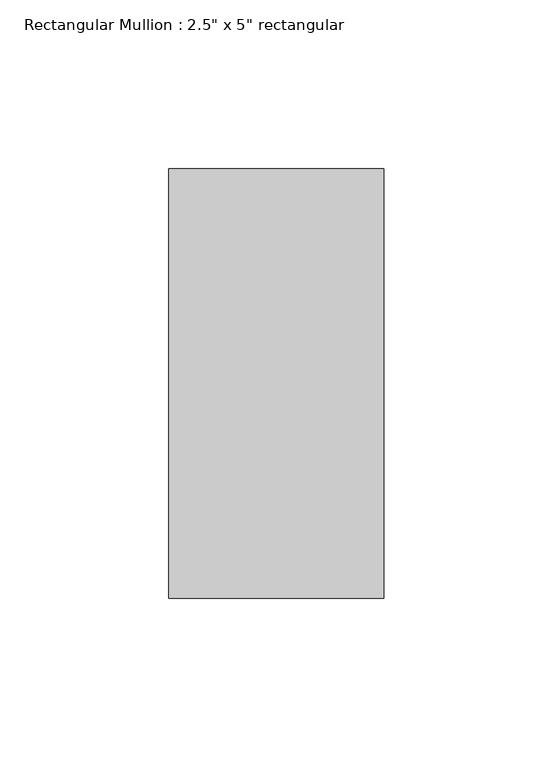
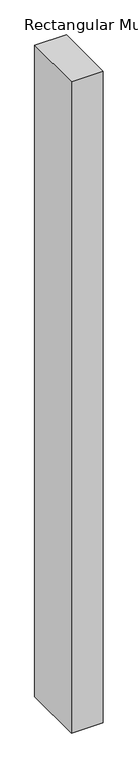
"""IFC4 building model written with IfcOpenShell, lengths in millimetres: member geometry."""

from ifc_helpers import new_model, si_unit, frame, origin, place, context, project, spatial, polyline, outline, extrude, source, transform, mapped, element, save


def member_79cc3911(model_context):
    return source(origin(), model_context, "Body", "SweptSolid", [
        extrude(outline(polyline([(0.0, 63.5), (0.0, -63.5), (-63.5, -63.5), (-63.5, 63.5), (0.0, 63.5)])), frame((0.0, 0.0, -1377.95), z_axis=(0.0, 0.0, 1.0), x_axis=(1.0, 0.0, 0.0)), (0.0, 0.0, 1.0), 1377.95),
    ])


if __name__ == "__main__":
    model = new_model("IFC4")
    model_context = context("Model", 3, world=origin())
    ifc_project = project(units=[si_unit("LENGTHUNIT", "METRE", prefix="MILLI")], contexts=[model_context])
    site = spatial("IfcSite", under=ifc_project)
    building = spatial("IfcBuilding", under=site)
    placement = place(None, origin())
    member_shape = member_79cc3911(model_context)
    element("IfcMember", 1, ObjectType="Rectangular Mullion : 2.5\" x 5\" rectangular", at=placement, inside=building, context=model_context, shape_type="MappedRepresentation", body=[
        mapped(member_shape, transform((0.0, 0.0, 0.0), x_axis=(1.0, 0.0, 0.0), y_axis=(0.0, 1.0, 0.0), z_axis=(0.0, 0.0, 1.0))),
    ])
    save(model, "model.ifc")

# Revit data of these elements
# Type "Rectangular Mullion : 2.5\" x 5\" rectangular"
#   built-in parameter 1007304 = 0.416667 (stored number, unit not read)
#   built-in parameter 1007301 = 0.104167 (stored number, unit not read)
#   built-in parameter 1007300 = 0.104167 (stored number, unit not read)
# Element 1 (IfcMember, "Rectangular Mullion : 2.5\" x 5\" rectangular")
#   Materials on its faces: "Aluminum"
# Materials
#   "Aluminum": class "Metal", colour RGB 247 247 247, transparency 0, Description = "Aluminum 6061", Cost = 0
